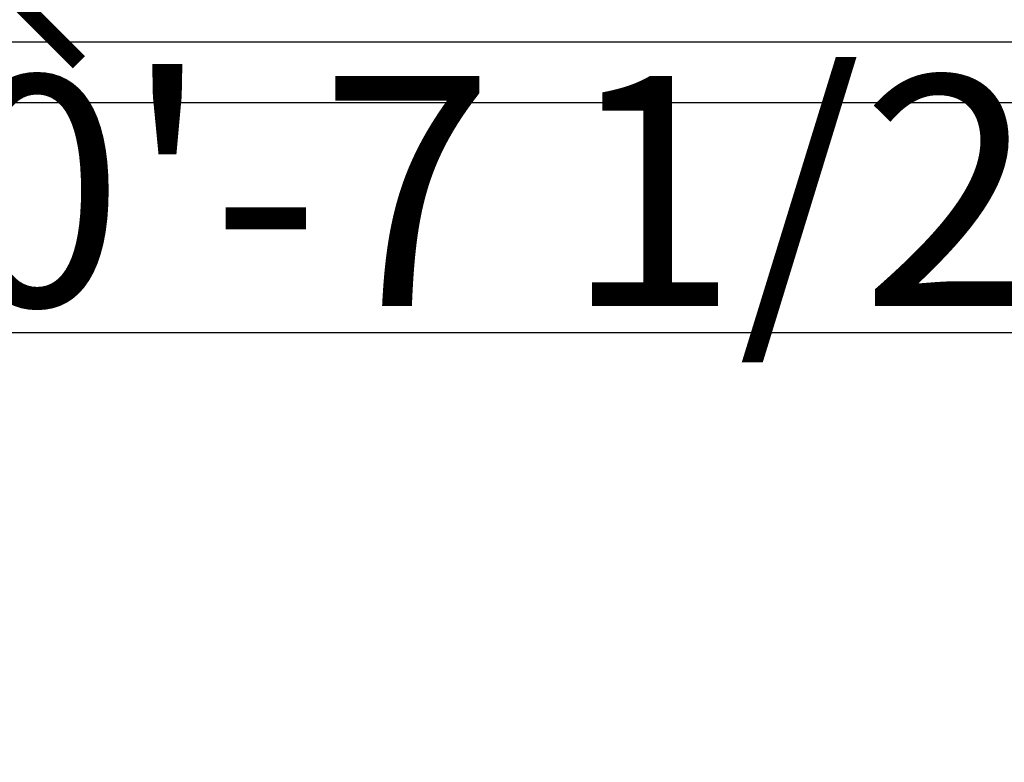
# Model space of a CAD drawing. Units: inches. Extents: x 2278 to 7495, y -71 to 1198.
# Tile 26 of 44: x 5101 to 5127, y 107 to 126. Entities that reach past the tile are written whole.
import ezdxf

# ---------------------------------------------------------------- set-up
doc = ezdxf.new("R2010")
doc.units = ezdxf.units.IN
doc.header["$MEASUREMENT"] = 0
doc.layers.add('A-ANNO-DIMS', color=2, linetype='Continuous', lineweight=18)
doc.layers.add('A-ELEV', color=7, linetype='Continuous', lineweight=25)
doc.styles.get("Standard").update_dxf_attribs({"font": 'arial.ttf'})
doc.dimstyles.get("Standard").update_dxf_attribs({"dimtxt": 6, "dimasz": 3, "dimexe": 0.18, "dimexo": 0.0625, "dimgap": 0.09, "dimtad": 0, "dimtih": 1, "dimtoh": 1, "dimdec": 0, "dimzin": 0, "dimdsep": 46, "dimlunit": 3, "dimtxsty": 'Standard', "dimblk": 'ARCHTICK', "dimcen": 0.09, "dimadec": 0, "dimazin": 0, "dimtfac": 1, "dimtdec": 0, "dimtofl": 0, "dimtmove": 0, "dimatfit": 3, "dimfxl": 1, "dimtolj": 1, "dimtzin": 0, "dimarcsym": 0})

# ---------------------------------------------------------------- blocks, each defined once
blk = doc.blocks.new('_ArchTick')
at = {"color": 0, "linetype": 'ByBlock', "const_width": 0.15}
blk.add_lwpolyline([(-0.5, -0.5), (0.5, 0.5)], dxfattribs=at)
blk = doc.blocks.new('*D59')
at = {"layer": 'A-ANNO-DIMS', "color": 0, "lineweight": -2, "transparency": 16777216}
for p, q in [((5096.589, 159.183), (5101.564, 159.183)), ((5101.384, 159.183), (5101.384, 146.185)), ((5101.384, 126.799), (5101.384, 139.796)), ((5096.589, 126.799), (5101.564, 126.799))]:
    blk.add_line(p, q, dxfattribs=at)
at = {"layer": 'Defpoints', "color": 0, "transparency": 16777216}
for p in [(5096.527, 159.183), (5101.384, 159.183), (5096.527, 126.799)]:
    blk.add_point(p, dxfattribs=at)
at = {"layer": 'A-ANNO-DIMS', "color": 0, "lineweight": -2, "transparency": 16777216, "xscale": 3, "yscale": 3, "zscale": 3}
for p, rotation in [((5101.384, 159.183), 90), ((5101.384, 126.799), 270)]:
    blk.add_blockref('_ArchTick', p, dxfattribs=dict(at, rotation=rotation))
at = {"layer": 'A-ANNO-DIMS', "color": 0, "transparency": 16777216, "insert": (5101.384, 142.991), "char_height": 6, "attachment_point": 5}
blk.add_mtext('\\A1;ORNATE BALUSTER 2\'-8 1/2" TYP.', dxfattribs=at)
blk = doc.blocks.new('*D60')
at = {"layer": 'A-ANNO-DIMS', "color": 0, "lineweight": -2, "transparency": 16777216}
for p, q in [((5088.787, 126.736), (5088.787, 121.761)), ((5096.527, 126.736), (5096.527, 121.761)), ((5088.787, 121.941), (5096.527, 121.941)), ((5096.527, 121.941), (5099.527, 121.941))]:
    blk.add_line(p, q, dxfattribs=at)
at = {"layer": 'Defpoints', "color": 0, "transparency": 16777216}
for p in [(5088.787, 126.799), (5096.527, 126.799), (5096.527, 121.941)]:
    blk.add_point(p, dxfattribs=at)
at = {"layer": 'A-ANNO-DIMS', "color": 0, "lineweight": -2, "transparency": 16777216, "xscale": 3, "yscale": 3, "zscale": 3, "rotation": 180}
blk.add_blockref('_ArchTick', (5088.787, 121.941), dxfattribs=at)
at = {"layer": 'A-ANNO-DIMS', "color": 0, "lineweight": -2, "transparency": 16777216, "xscale": 3, "yscale": 3, "zscale": 3}
blk.add_blockref('_ArchTick', (5096.527, 121.941), dxfattribs=at)
at = {"layer": 'A-ANNO-DIMS', "color": 0, "transparency": 16777216, "insert": (5124.894, 121.941), "char_height": 6, "attachment_point": 5}
blk.add_mtext('\\A1;0\'-7 1/2" TYP.', dxfattribs=at)
blk = doc.blocks.new('*D123')
at = {"layer": 'A-ANNO-DIMS', "color": 0, "lineweight": -2, "transparency": 16777216}
for p, q in [((4736.95, 340.157), (4736.95, -23.427)), ((5145.676, -1.81), (5145.676, -23.427)), ((4736.95, -23.247), (4923.929, -23.247)), ((5145.676, -23.247), (4958.697, -23.247))]:
    blk.add_line(p, q, dxfattribs=at)
at = {"layer": 'Defpoints', "color": 0, "transparency": 16777216}
for p in [(4736.95, 340.219), (5145.676, -1.747), (5145.676, -23.247)]:
    blk.add_point(p, dxfattribs=at)
at = {"layer": 'A-ANNO-DIMS', "color": 0, "lineweight": -2, "transparency": 16777216, "xscale": 3, "yscale": 3, "zscale": 3, "rotation": 180}
blk.add_blockref('_ArchTick', (4736.95, -23.247), dxfattribs=at)
at = {"layer": 'A-ANNO-DIMS', "color": 0, "lineweight": -2, "transparency": 16777216, "xscale": 3, "yscale": 3, "zscale": 3}
blk.add_blockref('_ArchTick', (5145.676, -23.247), dxfattribs=at)
at = {"layer": 'A-ANNO-DIMS', "color": 0, "transparency": 16777216, "insert": (4941.313, -23.247), "char_height": 6, "attachment_point": 5}
blk.add_mtext('\\A1;34\'-0 1/2"', dxfattribs=at)
blk = doc.blocks.new('*D131')
at = {"layer": 'A-ANNO-DIMS', "color": 0, "lineweight": -2, "transparency": 16777216}
for p, q in [((5096.176, 99.315), (5096.176, 361.899)), ((5145.676, 118.315), (5145.676, 361.899)), ((5096.176, 361.719), (5105.75, 361.719)), ((5145.676, 361.719), (5136.102, 361.719))]:
    blk.add_line(p, q, dxfattribs=at)
at = {"layer": 'Defpoints', "color": 0, "transparency": 16777216}
for p in [(5145.676, 361.719), (5145.676, 118.253), (5096.176, 99.253)]:
    blk.add_point(p, dxfattribs=at)
at = {"layer": 'A-ANNO-DIMS', "color": 0, "lineweight": -2, "transparency": 16777216, "xscale": 3, "yscale": 3, "zscale": 3, "rotation": 180}
blk.add_blockref('_ArchTick', (5096.176, 361.719), dxfattribs=at)
at = {"layer": 'A-ANNO-DIMS', "color": 0, "lineweight": -2, "transparency": 16777216, "xscale": 3, "yscale": 3, "zscale": 3}
blk.add_blockref('_ArchTick', (5145.676, 361.719), dxfattribs=at)
at = {"layer": 'A-ANNO-DIMS', "color": 0, "transparency": 16777216, "insert": (5120.926, 361.719), "char_height": 6, "attachment_point": 5}
blk.add_mtext('\\A1;4\'-1 1/2"', dxfattribs=at)
blk = doc.blocks.new('*D138')
at = {"layer": 'A-ANNO-DIMS', "color": 0, "lineweight": -2, "transparency": 16777216}
for p, q in [((5145.739, 118.253), (5167.754, 118.253)), ((5167.574, 118.253), (5167.574, 111.855)), ((5167.574, 99.253), (5167.574, 105.651)), ((5096.239, 99.253), (5167.754, 99.253))]:
    blk.add_line(p, q, dxfattribs=at)
at = {"layer": 'Defpoints', "color": 0, "transparency": 16777216}
for p in [(5145.676, 118.253), (5167.574, 118.253), (5096.176, 99.253)]:
    blk.add_point(p, dxfattribs=at)
at = {"layer": 'A-ANNO-DIMS', "color": 0, "lineweight": -2, "transparency": 16777216, "xscale": 3, "yscale": 3, "zscale": 3}
for p, rotation in [((5167.574, 118.253), 90), ((5167.574, 99.253), 270)]:
    blk.add_blockref('_ArchTick', p, dxfattribs=dict(at, rotation=rotation))
at = {"layer": 'A-ANNO-DIMS', "color": 0, "transparency": 16777216, "insert": (5167.574, 108.753), "char_height": 6, "attachment_point": 5}
blk.add_mtext('\\A1;1\'-7"', dxfattribs=at)
blk = doc.blocks.new('*D139')
at = {"layer": 'A-ANNO-DIMS', "color": 0, "lineweight": -2, "transparency": 16777216}
for p, q in [((5092.239, 160.253), (5167.754, 160.253)), ((5167.574, 160.253), (5167.574, 142.408)), ((5167.574, 118.253), (5167.574, 136.097)), ((5145.739, 118.253), (5167.754, 118.253))]:
    blk.add_line(p, q, dxfattribs=at)
at = {"layer": 'Defpoints', "color": 0, "transparency": 16777216}
for p in [(5092.176, 160.253), (5167.574, 160.253), (5145.676, 118.253)]:
    blk.add_point(p, dxfattribs=at)
at = {"layer": 'A-ANNO-DIMS', "color": 0, "lineweight": -2, "transparency": 16777216, "xscale": 3, "yscale": 3, "zscale": 3}
for p, rotation in [((5167.574, 160.253), 90), ((5167.574, 118.253), 270)]:
    blk.add_blockref('_ArchTick', p, dxfattribs=dict(at, rotation=rotation))
at = {"layer": 'A-ANNO-DIMS', "color": 0, "transparency": 16777216, "insert": (5167.574, 139.253), "char_height": 6, "attachment_point": 5}
blk.add_mtext('\\A1;3\'-6"', dxfattribs=at)

msp = doc.modelspace()

# ---------------------------------------------------------------- linework, layer by layer
at = {"layer": 'A-ELEV'}
for p, q in [((5145.676, 125.821), (5066.016, 125.821)), ((4874.676, 124.253), (5145.676, 124.253)), ((4874.676, 118.253), (5145.676, 118.253))]:
    msp.add_line(p, q, dxfattribs=at)

# ---------------------------------------------------------------- dimensions: what is measured, and where the dimension line sits
at = {"layer": 'A-ANNO-DIMS'}
for base, p1, p2, picture, middle in [((5145.676, 361.719), (5096.176, 99.253), (5145.676, 118.253), '*D131', (5120.926, 361.719)), ((5145.676, -23.247), (4736.95, 340.219), (5145.676, -1.747), '*D123', (4941.313, -23.247))]:
    dim = msp.add_linear_dim(base=base, p1=p1, p2=p2, dimstyle='Standard', override={"dimdec": 1, "dimlfac": 1, "dimrnd": 0, "dimzin": 1, "dimdsep": 46, "dimlunit": 4, "dimfrac": 2}, dxfattribs=at)
    dim.commit()
    dim.dimension.update_dxf_attribs({"geometry": picture, "text_midpoint": middle})
dim = msp.add_linear_dim(base=(5101.384, 159.183), p1=(5096.527, 126.799), p2=(5096.527, 159.183), angle=90, text='ORNATE BALUSTER <> TYP.', dimstyle='Standard', override={"dimdec": 1, "dimrnd": 0, "dimzin": 1, "dimlunit": 4, "dimfrac": 2}, dxfattribs=at)
dim.commit()
dim.dimension.update_dxf_attribs({"geometry": '*D59', "text_midpoint": (5101.384, 142.991)})
for base, p1, p2, picture, middle in [((5167.574, 160.253), (5145.676, 118.253), (5092.176, 160.253), '*D139', (5167.574, 139.253)), ((5167.574, 118.253), (5096.176, 99.253), (5145.676, 118.253), '*D138', (5167.574, 108.753))]:
    dim = msp.add_linear_dim(base=base, p1=p1, p2=p2, angle=90, dimstyle='Standard', override={"dimdec": 1, "dimlfac": 1, "dimrnd": 0, "dimzin": 1, "dimdsep": 46, "dimlunit": 4, "dimfrac": 2}, dxfattribs=at)
    dim.commit()
    dim.dimension.update_dxf_attribs({"geometry": picture, "text_midpoint": middle})
dim = msp.add_linear_dim(base=(5096.527, 121.941), p1=(5088.787, 126.799), p2=(5096.527, 126.799), text='<> TYP.', dimstyle='Standard', override={"dimdec": 1, "dimrnd": 0, "dimzin": 1, "dimlunit": 4, "dimfrac": 2}, dxfattribs=at)
dim.commit()
dim.dimension.update_dxf_attribs({"geometry": '*D60', "text_midpoint": (5124.894, 121.941)})

doc.saveas('drawing.dxf')
